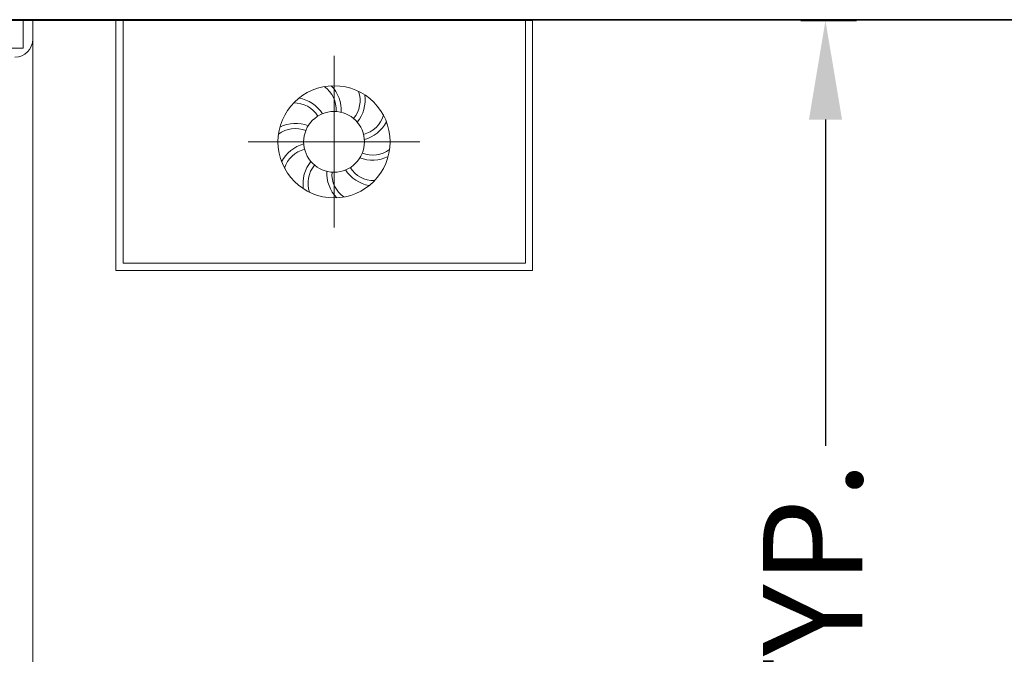
# Model space of a CAD drawing. Units: inches. Extents: x -638 to 186, y -762 to 59.
# Tile 28 of 31: x -66 to -26, y -77 to -51. Entities that reach past the tile are written whole.
import ezdxf

# ---------------------------------------------------------------- set-up
doc = ezdxf.new("R2010")
doc.units = ezdxf.units.IN
for name, color, linetype, lineweight in [('A-ANNO-DIMS', 2, 'Continuous', 18), ('furn', 8, 'Continuous', 13), ('wall', 7, 'Continuous', 35)]:
    doc.layers.add(name, color=color, linetype=linetype, lineweight=lineweight)
doc.styles.get("Standard").update_dxf_attribs({"font": 'arial.ttf'})
doc.dimstyles.new('ISO-25', dxfattribs={"dimtxt": 4, "dimasz": 4, "dimexe": 1.25, "dimexo": 0.625, "dimtad": 0, "dimlunit": 4, "dimtxsty": 'Standard', "dimcen": 2.5, "dimclrt": 256, "dimadec": 0, "dimazin": 0, "dimtfac": 1, "dimtmove": 0, "dimatfit": 3, "dimfxl": 1, "dimfxlon": 1, "dimarcsym": 0})

# ---------------------------------------------------------------- blocks, each defined once
blk = doc.blocks.new('BED-DOUBLE-WITH-NIGHTSTANDS')
for p, q in [((0, 59.951), (78.699, 59.951)), ((58.161, 59.951), (58.161, 58.826)), ((58.548, 11.244), (58.548, 59.951)), ((61.904, 59.951), (61.904, 49.874)), ((62.191, 59.951), (62.191, 50.162)), ((78.411, 50.162), (78.411, 59.951)), ((78.699, 49.874), (78.699, 59.951)), ((58.161, 58.826), (20.398, 58.826)), ((70.694, 51.596), (70.694, 58.516)), ((74.154, 55.056), (67.234, 55.056)), ((62.191, 50.162), (78.411, 50.162)), ((61.904, 49.874), (78.699, 49.874))]:
    blk.add_line(p, q)
for radius in [2.26, 1.225]:
    blk.add_circle((70.694, 55.056), radius)
for centre, radius, start, end in [((57.828, 59.188), 0.72, 270, 0), ((69.67, 56.366), 1.108, 355.462, 55.6998), ((69.537, 56.308), 1.452, 357.5103, 43.83), ((69.022, 55.389), 1.452, 33.5103, 79.83), ((70.636, 56.718), 1.108, 319.462, 19.6998), ((70.494, 56.749), 1.452, 321.5103, 7.83), ((69.096, 55.514), 1.108, 31.462, 91.6998), ((71.623, 56.435), 1.108, 283.462, 343.6998), ((69.132, 54.487), 1.108, 67.462, 127.6998), ((69.146, 54.343), 1.452, 69.5103, 115.83), ((71.527, 56.544), 1.452, 285.5103, 331.83), ((69.861, 53.569), 1.452, 105.5103, 151.83), ((69.765, 53.678), 1.108, 103.462, 163.6998), ((72.242, 55.77), 1.452, 249.5103, 295.83), ((72.256, 55.625), 1.108, 247.462, 307.6998), ((70.894, 53.363), 1.452, 141.5103, 187.83), ((70.753, 53.395), 1.108, 139.462, 199.6998), ((72.292, 54.599), 1.108, 211.462, 271.6998), ((71.851, 53.804), 1.452, 177.5103, 223.83), ((71.718, 53.747), 1.108, 175.462, 235.6998), ((72.366, 54.723), 1.452, 213.5103, 259.83)]:
    blk.add_arc(centre, radius, start, end)
blk = doc.blocks.new('*D28')
at = {"layer": 'A-ANNO-DIMS', "color": 0, "lineweight": -2, "transparency": 16777216}
for p, q in [((-34.121, -51.062), (-31.871, -51.062)), ((-33.121, -55.062), (-33.121, -68.221)), ((-33.121, -107.013), (-33.121, -93.853)), ((-34.121, -111.013), (-31.871, -111.013))]:
    blk.add_line(p, q, dxfattribs=at)
at = {"layer": 'A-ANNO-DIMS', "color": 0, "lineweight": 30, "transparency": 16777216}
for points in [[(-33.787, -55.062), (-32.454, -55.062), (-33.121, -51.062)], [(-33.787, -107.013), (-32.454, -107.013), (-33.121, -111.013)]]:
    blk.add_solid(points, dxfattribs=at)
at = {"layer": 'Defpoints', "color": 0, "lineweight": 30, "transparency": 16777216}
for p in [(-44.925, -51.062), (-33.121, -51.062), (-44.925, -111.013)]:
    blk.add_point(p, dxfattribs=at)
at = {"layer": 'A-ANNO-DIMS', "transparency": 16777216, "insert": (-33.121, -81.037), "char_height": 4, "attachment_point": 5, "rotation": 90}
blk.add_mtext('5\'-0" TYP.', dxfattribs=at)

msp = doc.modelspace()

# ---------------------------------------------------------------- linework, layer by layer
at = {"layer": 'wall'}
msp.add_line((-160.526, -51.033), (1.474, -51.033), dxfattribs=at)
msp.add_line((-160.526, -51.033), (1.474, -51.033), dxfattribs=at)

# ---------------------------------------------------------------- block references
at = {"layer": 'furn'}
msp.add_blockref('BED-DOUBLE-WITH-NIGHTSTANDS', (-123.625, -111.013), dxfattribs=at)

# ---------------------------------------------------------------- dimensions: what is measured, and where the dimension line sits
at = {"layer": 'A-ANNO-DIMS'}
dim = msp.add_linear_dim(base=(-33.121, -51.062), p1=(-44.925, -111.013), p2=(-44.925, -51.062), angle=90, text='<> TYP.', dimstyle='ISO-25', override={"dimdec": 1, "dimlfac": 1, "dimrnd": 0, "dimzin": 1, "dimdsep": 46, "dimlunit": 4, "dimfrac": 2}, dxfattribs=at)
dim.commit()
dim.dimension.update_dxf_attribs({"geometry": '*D28', "text_midpoint": (-33.121, -81.037)})

doc.saveas('drawing.dxf')
